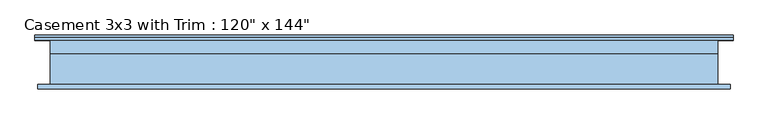
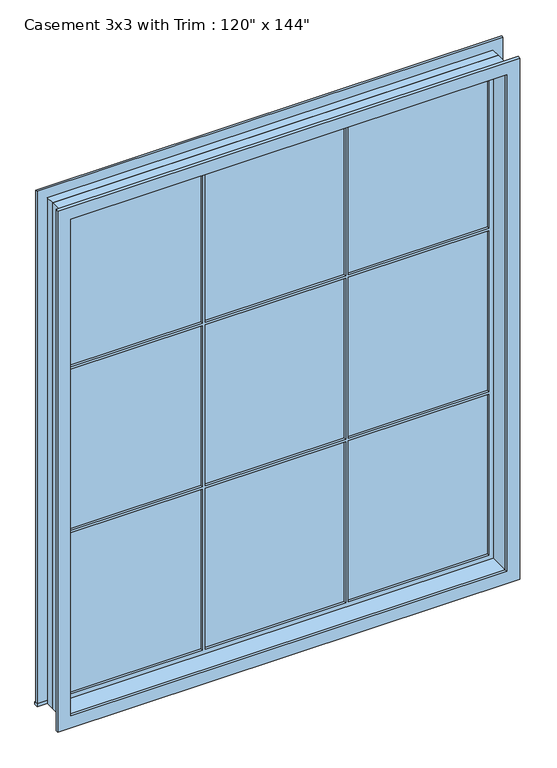
"""IFC4 building model written with IfcOpenShell, lengths in millimetres: window geometry."""

from ifc_helpers import new_model, si_unit, frame, origin, place, context, project, spatial, polyline, outline, extrude, source, transform, mapped, element, save


def window_cae7f124(model_context):
    return source(origin(), model_context, "Body", "SweptSolid", [
        extrude(outline(polyline([(-1593.85, 127.0), (1593.85, 127.0), (1593.85, 101.6), (-1593.85, 101.6), (-1593.85, 127.0)])), frame((0.0, 0.0, 5486.4), z_axis=(0.0, 0.0, 1.0), x_axis=(1.0, 0.0, 0.0)), (0.0, 0.0, 1.0), 19.05),
        extrude(outline(polyline([(9124.95, -1504.95), (9124.95, 1504.95), (5505.45, 1504.95), (5505.45, 1593.85), (9213.85, 1593.85), (9213.85, -1593.85), (5505.45, -1593.85), (5505.45, -1504.95), (9124.95, -1504.95)])), frame((0.0, 101.6, 0.0), z_axis=(0.0, 1.0, 0.0), x_axis=(0.0, 0.0, 1.0)), (0.0, 0.0, 1.0), 12.7),
        extrude(outline(polyline([(499.5333333, 66.675), (1460.5, 66.675), (1460.5, 53.975), (499.5333333, 53.975), (499.5333333, 66.675)])), frame((0.0, 0.0, 7916.3333333), z_axis=(0.0, 0.0, 1.0), x_axis=(1.0, 0.0, 0.0)), (0.0, 0.0, 1.0), 1164.1666667),
        extrude(outline(polyline([(-480.4833333, 66.675), (480.4833333, 66.675), (480.4833333, 53.975), (-480.4833333, 53.975), (-480.4833333, 66.675)])), frame((0.0, 0.0, 7916.3333333), z_axis=(0.0, 0.0, 1.0), x_axis=(1.0, 0.0, 0.0)), (0.0, 0.0, 1.0), 1164.1666667),
        extrude(outline(polyline([(-1460.5, 66.675), (-499.5333333, 66.675), (-499.5333333, 53.975), (-1460.5, 53.975), (-1460.5, 66.675)])), frame((0.0, 0.0, 7916.3333333), z_axis=(0.0, 0.0, 1.0), x_axis=(1.0, 0.0, 0.0)), (0.0, 0.0, 1.0), 1164.1666667),
        extrude(outline(polyline([(-1460.5, 66.675), (-499.5333333, 66.675), (-499.5333333, 53.975), (-1460.5, 53.975), (-1460.5, 66.675)])), frame((0.0, 0.0, 6733.1166667), z_axis=(0.0, 0.0, 1.0), x_axis=(1.0, 0.0, 0.0)), (0.0, 0.0, 1.0), 1164.1666667),
        extrude(outline(polyline([(-480.4833333, 66.675), (480.4833333, 66.675), (480.4833333, 53.975), (-480.4833333, 53.975), (-480.4833333, 66.675)])), frame((0.0, 0.0, 6733.1166667), z_axis=(0.0, 0.0, 1.0), x_axis=(1.0, 0.0, 0.0)), (0.0, 0.0, 1.0), 1164.1666667),
        extrude(outline(polyline([(499.5333333, 66.675), (1460.5, 66.675), (1460.5, 53.975), (499.5333333, 53.975), (499.5333333, 66.675)])), frame((0.0, 0.0, 6733.1166667), z_axis=(0.0, 0.0, 1.0), x_axis=(1.0, 0.0, 0.0)), (0.0, 0.0, 1.0), 1164.1666667),
        extrude(outline(polyline([(499.5333333, 66.675), (1460.5, 66.675), (1460.5, 53.975), (499.5333333, 53.975), (499.5333333, 66.675)])), frame((0.0, 0.0, 5549.9), z_axis=(0.0, 0.0, 1.0), x_axis=(1.0, 0.0, 0.0)), (0.0, 0.0, 1.0), 1164.1666667),
        extrude(outline(polyline([(-480.4833333, 66.675), (480.4833333, 66.675), (480.4833333, 53.975), (-480.4833333, 53.975), (-480.4833333, 66.675)])), frame((0.0, 0.0, 5549.9), z_axis=(0.0, 0.0, 1.0), x_axis=(1.0, 0.0, 0.0)), (0.0, 0.0, 1.0), 1164.1666667),
        extrude(outline(polyline([(-1460.5, 66.675), (-499.5333333, 66.675), (-499.5333333, 53.975), (-1460.5, 53.975), (-1460.5, 66.675)])), frame((0.0, 0.0, 5549.9), z_axis=(0.0, 0.0, 1.0), x_axis=(1.0, 0.0, 0.0)), (0.0, 0.0, 1.0), 1164.1666667),
        extrude(outline(polyline([(9201.15, 1581.15), (9201.15, -1581.15), (5429.25, -1581.15), (5429.25, 1581.15), (9201.15, 1581.15)]), holes=[polyline([(9112.25, 1492.25), (5518.15, 1492.25), (5518.15, -1492.25), (9112.25, -1492.25), (9112.25, 1492.25)])]), frame((0.0, -120.65, 0.0), z_axis=(0.0, 1.0, 0.0), x_axis=(0.0, 0.0, 1.0)), (0.0, 0.0, 1.0), 19.05),
        extrude(outline(polyline([(9124.95, -1504.95), (5505.45, -1504.95), (5505.45, 1504.95), (9124.95, 1504.95), (9124.95, -1504.95)]), holes=[polyline([(9080.5, -499.5333333), (7916.3333333, -499.5333333), (7916.3333333, -1460.5), (9080.5, -1460.5), (9080.5, -499.5333333)]), polyline([(7897.2833333, -499.5333333), (6733.1166667, -499.5333333), (6733.1166667, -1460.5), (7897.2833333, -1460.5), (7897.2833333, -499.5333333)]), polyline([(6714.0666667, -499.5333333), (5549.9, -499.5333333), (5549.9, -1460.5), (6714.0666667, -1460.5), (6714.0666667, -499.5333333)]), polyline([(9080.5, 480.4833333), (7916.3333333, 480.4833333), (7916.3333333, -480.4833333), (9080.5, -480.4833333), (9080.5, 480.4833333)]), polyline([(7897.2833333, 480.4833333), (6733.1166667, 480.4833333), (6733.1166667, -480.4833333), (7897.2833333, -480.4833333), (7897.2833333, 480.4833333)]), polyline([(6714.0666667, 480.4833333), (5549.9, 480.4833333), (5549.9, -480.4833333), (6714.0666667, -480.4833333), (6714.0666667, 480.4833333)]), polyline([(9080.5, 1460.5), (7916.3333333, 1460.5), (7916.3333333, 499.5333333), (9080.5, 499.5333333), (9080.5, 1460.5)]), polyline([(7897.2833333, 1460.5), (6733.1166667, 1460.5), (6733.1166667, 499.5333333), (7897.2833333, 499.5333333), (7897.2833333, 1460.5)]), polyline([(6714.0666667, 1460.5), (5549.9, 1460.5), (5549.9, 499.5333333), (6714.0666667, 499.5333333), (6714.0666667, 1460.5)])]), frame((0.0, 38.1, 0.0), z_axis=(0.0, 1.0, 0.0), x_axis=(0.0, 0.0, 1.0)), (0.0, 0.0, 1.0), 44.45),
        extrude(outline(polyline([(9144.0, -1524.0), (5486.4, -1524.0), (5486.4, 1524.0), (9144.0, 1524.0), (9144.0, -1524.0)]), holes=[polyline([(9112.25, -1492.25), (9112.25, 1492.25), (5518.15, 1492.25), (5518.15, -1492.25), (9112.25, -1492.25)])]), frame((0.0, -101.6, 0.0), z_axis=(0.0, 1.0, 0.0), x_axis=(0.0, 0.0, 1.0)), (0.0, 0.0, 1.0), 139.7),
        extrude(outline(polyline([(9144.0, 1524.0), (9144.0, -1524.0), (5486.4, -1524.0), (5486.4, 1524.0), (9144.0, 1524.0)]), holes=[polyline([(9124.95, 1504.95), (5505.45, 1504.95), (5505.45, -1504.95), (9124.95, -1504.95), (9124.95, 1504.95)])]), frame((0.0, 38.1, 0.0), z_axis=(0.0, 1.0, 0.0), x_axis=(0.0, 0.0, 1.0)), (0.0, 0.0, 1.0), 63.5),
    ])


if __name__ == "__main__":
    model = new_model("IFC4")
    model_context = context("Model", 3, world=origin())
    ifc_project = project(units=[si_unit("LENGTHUNIT", "METRE", prefix="MILLI")], contexts=[model_context])
    site = spatial("IfcSite", under=ifc_project)
    building = spatial("IfcBuilding", under=site)
    placement = place(None, origin())
    window_shape = window_cae7f124(model_context)
    element("IfcWindow", 1, ObjectType="Casement 3x3 with Trim : 120\" x 144\"", at=placement, inside=building, context=model_context, shape_type="MappedRepresentation", body=[
        mapped(window_shape, transform((0.0, 0.0, 0.0), x_axis=(1.0, 0.0, 0.0), y_axis=(0.0, 1.0, 0.0), z_axis=(0.0, 0.0, 1.0))),
    ])
    save(model, "model.ifc")

# Revit data of these elements
# Type "Casement 3x3 with Trim : 120\" x 144\""
#   Type Mark = "10"
#   Construction Type Id = "GSP4R"
#   Assembly Code = "B2020100"
#   Analytic Construction = "1/8 in Pilkington single glazing"
#   Visual Light Transmittance = 0.9
#   Solar Heat Gain Coefficient = 0.78
#   Heat Transfer Coefficient (U) = 0.6496 BTU/(h·ft²·°F)
#   Height = 12' - 0"
#   Default Sill Height = 18' - 0"
#   Trim Projection - Ext. = 0' - 0 1/2"
#   Trim Projection - Int. = 0' - 0 3/4"
#   Trim Width - Exterior = 0' - 3 1/2"
#   Trim Width - Interior = 0' - 3 1/2"
#   Width = 10' - 0"
#   Window Inset = 0' - 0 3/4"
#   Define Thermal Properties by = 1
#   Glass Pane Material = Glass
#   Sash Material = Sash
#   Trim Exterior Material = Trim
#   Trim Interior Material = Trim
#   Wall Closure = (empty or 0)
# Element 1 (IfcWindow, "Casement 3x3 with Trim : 120\" x 144\"")
#   Materials on its faces: "Sash", "Glass", "Trim"
# Materials
#   "Glass": class "Glass", colour RGB 0 128 192, transparency 0.75, Description = "Soda Lime Glass", Cost = 0
#   "Sash": class "Wood", colour RGB 224 178 126, transparency 0
#   "Trim": class "Wood", colour RGB 224 178 126, transparency 0
